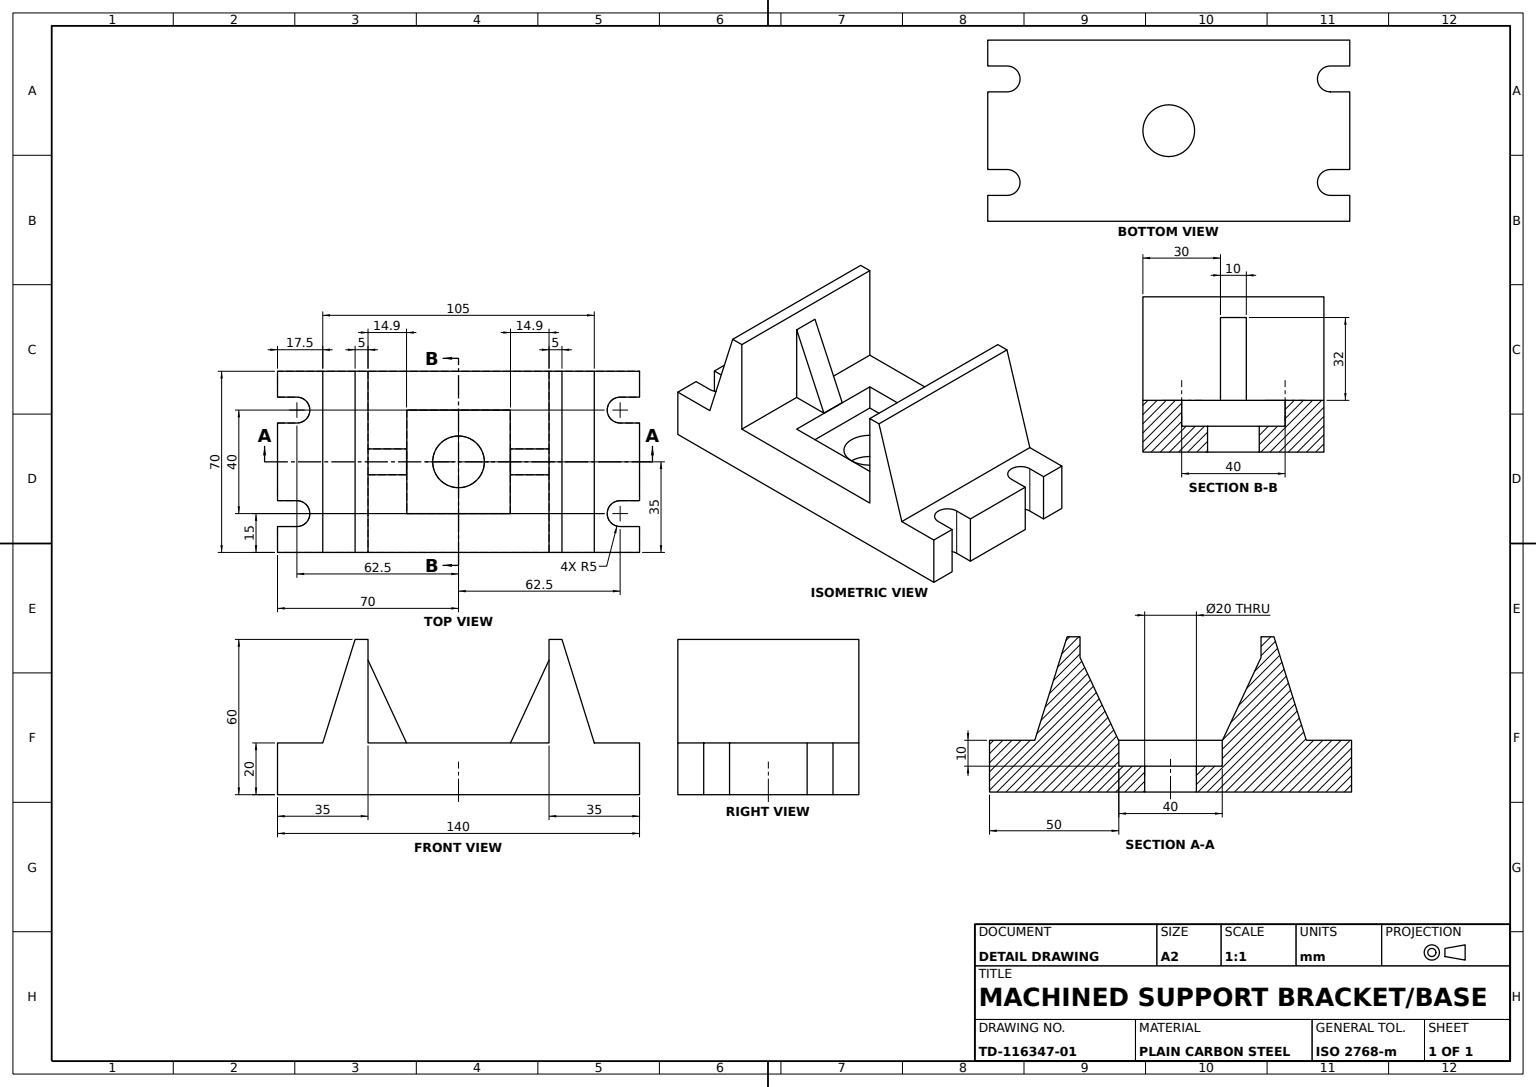
from build123d import *

# Parameters (mm, degrees)
BASE_PLATE_140X70X20_DEPTH   = 20
CENTRE_HOLE_SKETCH_R         = 10
CENTRE_HOLE_20_DEPTH         = 20
CENTRE_POCKET_SKETCH_W       = 40
CENTRE_POCKET_SKETCH_H       = 40
CENTRE_POCKET_40X40X10_DEPTH = 10
V_BLOCK_UPRIGHTS_DEPTH       = 70
GUSSET_RIB_DEPTH             = 5


with BuildPart() as part:
    # Base Plate Sketch → Base Plate 140x70x20 (new body)
    with BuildSketch(Plane(origin=(0, 0, 0), x_dir=(1, 0, 0), z_dir=(0, 1, 0))):
        with BuildLine():
            Line((-70, 25), (-62.5, 25))
            ThreePointArc((-62.5, 25), (-57.5, 20), (-62.5, 15))
            Line((-62.5, 15), (-70, 15))
            Line((-70, 15), (-70, -15))
            Line((-70, -15), (-62.5, -15))
            ThreePointArc((-62.5, -15), (-57.5, -20), (-62.5, -25))
            Line((-62.5, -25), (-70, -25))
            Line((-70, -25), (-70, -35))
            Line((-70, -35), (70, -35))
            Line((70, -35), (70, -25))
            Line((70, -25), (62.5, -25))
            ThreePointArc((62.5, -25), (57.5, -20), (62.5, -15))
            Line((62.5, -15), (70, -15))
            Line((70, -15), (70, 15))
            Line((70, 15), (62.5, 15))
            ThreePointArc((62.5, 15), (57.5, 20), (62.5, 25))
            Line((62.5, 25), (70, 25))
            Line((70, 25), (70, 35))
            Line((70, 35), (-70, 35))
            Line((-70, 35), (-70, 25))
        make_face()
    extrude(amount=BASE_PLATE_140X70X20_DEPTH)

    # Centre Hole Sketch → Centre Hole Ø20 (cut)
    with BuildSketch(Plane(origin=(0, 20, 0), x_dir=(1, 0, 0), z_dir=(0, 1, 0))):
        with Locations(Location((0, 0, 0), (0, 0, 270))):
            Circle(CENTRE_HOLE_SKETCH_R)
    extrude(amount=-CENTRE_HOLE_20_DEPTH, mode=Mode.SUBTRACT)

    # Centre Pocket Sketch → Centre Pocket 40x40x10 (cut)
    with BuildSketch(Plane(origin=(0, 20, 0), x_dir=(1, 0, 0), z_dir=(0, 1, 0))):
        Rectangle(CENTRE_POCKET_SKETCH_W, CENTRE_POCKET_SKETCH_H)
    extrude(amount=-CENTRE_POCKET_40X40X10_DEPTH, mode=Mode.SUBTRACT)

    # V-Block Uprights Sketch → V-Block Uprights (add)
    with BuildSketch(Plane.XY.offset(35)):
        Polygon((-40, 60), (-52.5, 20), (-35, 20), (-35, 60), align=None)
        Polygon((35, 60), (35, 20), (52.5, 20), (40, 60), align=None)
    extrude(amount=-V_BLOCK_UPRIGHTS_DEPTH)

    # Gusset Rib Sketch → Gusset Rib (add, symmetric)
    with BuildSketch(Plane.XY):
        Polygon((-20.102951906, 20), (-35, 20), (-35, 52), align=None)
        Polygon((20.1, 20), (35, 52), (35, 20), align=None)
    extrude(amount=GUSSET_RIB_DEPTH, both=True)


solid = part.part
